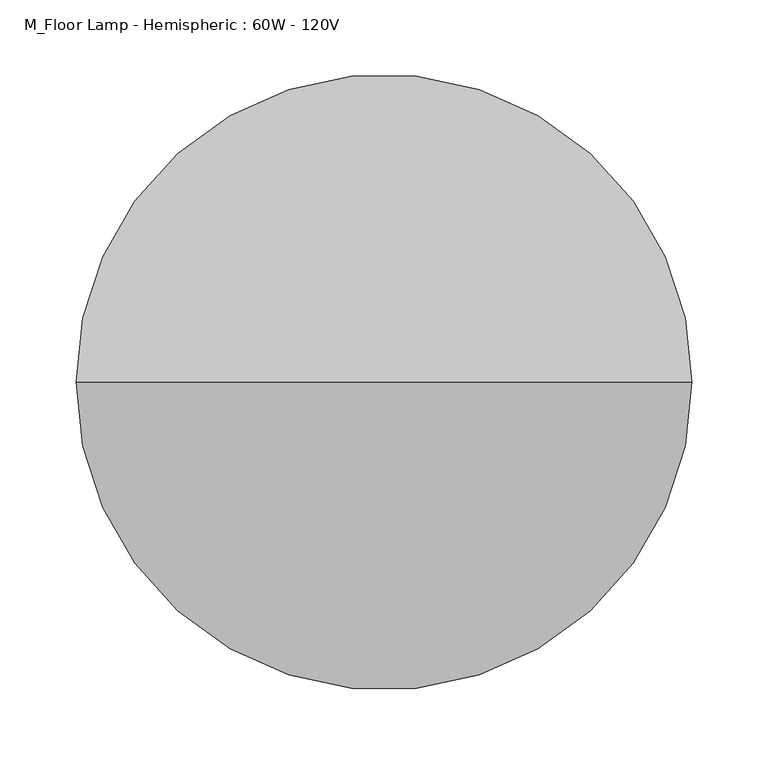
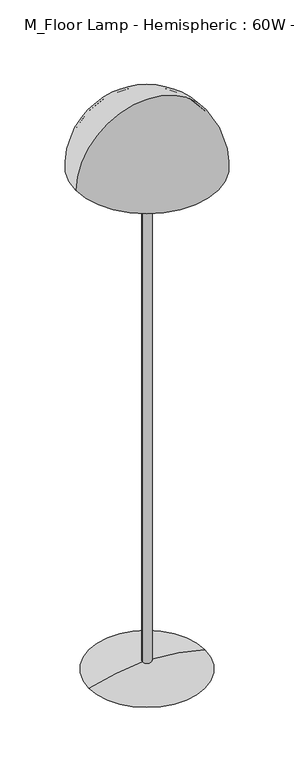
"""IFC4 building model written with IfcOpenShell, lengths in millimetres: light fixture geometry, M_Floor Lamp - Hemispheric : 60W - 120V."""

from ifc_helpers import new_model, si_unit, point, frame, origin, origin_with_axes, origin_2d, place, context, project, spatial, polyline, circle_curve, ellipse_curve, trimmed, segment, composite_curve, outline, extrude, source, transform, mapped, element, save
from ifc_brep_helpers import plane_surface, revolved_surface, advanced_brep


def m_floor_lamp_hemispheric_60w_120v_4a08ccbb(model_context):
    return source(origin(), model_context, "Body", "SolidModel", [
        extrude(outline(composite_curve([segment(trimmed(circle_curve(origin_2d(), 12.7), [point((-12.7, 0.0))], [point((12.7, 0.0))], False, "CARTESIAN"), True, "CONTINUOUS"), segment(trimmed(circle_curve(origin_2d(), 12.7), [point((12.7, 0.0))], [point((-12.7, 0.0))], False, "CARTESIAN"), True, "CONTINUOUS")], self_intersect=False)), frame((0.0, 0.0, 25.4), z_axis=(0.0, 0.0, 1.0), x_axis=(1.0, 0.0, 0.0)), (0.0, 0.0, 1.0), 1524.0),
        advanced_brep(
        [(-165.1, 0.0, 0.0), (165.1, 0.0, 0.0), (12.7, 0.0, 0.0), (-12.7, 0.0, 0.0), (-12.7, 0.0, 25.4), (12.7, 0.0, 25.4)],
        [
            (0, 1, circle_curve(frame((0.0, 0.0, 0.0), z_axis=(0.0, 0.0, -1.0), x_axis=(1.0, 0.0, 0.0)), 165.1)),
            (1, 2),
            (2, 3, circle_curve(origin_with_axes(), 12.7)),
            (3, 0),
            (1, 0, circle_curve(frame((0.0, 0.0, 0.0), z_axis=(0.0, 0.0, -1.0), x_axis=(1.0, 0.0, 0.0)), 165.1)),
            (3, 2, circle_curve(origin_with_axes(), 12.7)),
            (4, 5, circle_curve(frame((0.0, 0.0, 25.4), z_axis=(0.0, 0.0, -1.0), x_axis=(1.0, 0.0, 0.0)), 12.7)),
            (5, 1, circle_curve(frame((-10.5405788, 0.0, -583.9434729), z_axis=(0.0, 1.0, 0.0), x_axis=(1.0, 0.0, 0.0)), 609.7865138)),
            (0, 4, circle_curve(frame((10.5405788, 0.0, -583.9434729), z_axis=(0.0, 1.0, 0.0), x_axis=(-1.0, 0.0, 0.0)), 609.7865138)),
            (5, 4, circle_curve(frame((0.0, 0.0, 25.4), z_axis=(0.0, 0.0, -1.0), x_axis=(1.0, 0.0, 0.0)), 12.7)),
            (2, 5),
            (4, 3),
        ],
        [
            plane_surface(frame((0.0, 0.0, 0.0), z_axis=(0.0, 0.0, -1.0), x_axis=(1.0, 0.0, 0.0))),
            revolved_surface(trimmed(ellipse_curve(frame((-10.5405788, 0.0, -583.9434729), z_axis=(0.0, -1.0, 0.0), x_axis=(1.0, 0.0, 0.0)), 609.7865138, 609.7865138), [point((165.1, 0.0, 0.0))], [point((12.7, 0.0, 25.4))], True, "CARTESIAN"), (0.0, 0.0, 127.0), (0.0, 0.0, 1.0)),
            revolved_surface(polyline([(12.7, 0.0, 25.400000000000006), (12.7, 0.0, 0.0)]), (0.0, 0.0, 127.0), (0.0, 0.0, 1.0)),
        ],
        [
            (0, [[1, 2, 3, 4]]),
            (0, [[5, -4, 6, -2]]),
            (1, [[7, 8, -1, 9]]),
            (1, [[10, -9, -5, -8]]),
            (2, [[-3, 11, -7, 12]]),
            (2, [[-6, -12, -10, -11]]),
        ],
    ),
        advanced_brep(
        [(-197.591573, 0.0, 1510.4133868), (197.591573, 0.0, 1510.4133868), (0.0, 0.0, 1707.4075084), (-202.3305676, 0.0, 1510.4133868), (202.3305676, 0.0, 1510.4133868), (0.0, 0.0, 1713.4837615)],
        [
            (0, 1, circle_curve(frame((0.0, 0.0, 1510.4133868), z_axis=(0.0, 0.0, -1.0), x_axis=(1.0, 0.0, 0.0)), 197.591573)),
            (1, 2, circle_curve(frame((0.7416268, 0.0, 1510.5589055), z_axis=(0.0, -1.0, 0.0), x_axis=(1.0, 0.0, 0.0)), 196.85)),
            (2, 0, circle_curve(frame((-0.7416268, 0.0, 1510.5589055), z_axis=(0.0, -1.0, 0.0), x_axis=(-1.0, 0.0, 0.0)), 196.85)),
            (1, 0, circle_curve(frame((0.0, 0.0, 1510.4133868), z_axis=(0.0, 0.0, -1.0), x_axis=(1.0, 0.0, 0.0)), 197.591573)),
            (3, 4, circle_curve(frame((0.0, 0.0, 1510.4133868), z_axis=(0.0, 0.0, -1.0), x_axis=(1.0, 0.0, 0.0)), 202.3305676)),
            (4, 1),
            (0, 3),
            (4, 3, circle_curve(frame((0.0, 0.0, 1510.4133868), z_axis=(0.0, 0.0, -1.0), x_axis=(1.0, 0.0, 0.0)), 202.3305676)),
            (5, 4, circle_curve(frame((-0.8693923, 0.0, 1510.2856214), z_axis=(0.0, 1.0, 0.0), x_axis=(1.0, 0.0, 0.0)), 203.2)),
            (3, 5, circle_curve(frame((0.8693923, 0.0, 1510.2856214), z_axis=(0.0, 1.0, 0.0), x_axis=(-1.0, 0.0, 0.0)), 203.2)),
        ],
        [
            revolved_surface(trimmed(ellipse_curve(frame((0.7416268, 0.0, 1510.5589055), z_axis=(0.0, 1.0, 0.0), x_axis=(1.0, 0.0, 0.0)), 196.85, 196.85), [point((0.0, 0.0, 1707.4075084))], [point((197.591573, 0.0, 1510.4133868))], True, "CARTESIAN"), (0.0, 0.0, 1815.2133868), (0.0, 0.0, 1.0)),
            plane_surface(frame((0.0, 0.0, 1510.4133868), z_axis=(0.0, 0.0, -1.0), x_axis=(1.0, 0.0, 0.0))),
            revolved_surface(trimmed(ellipse_curve(frame((-0.8693923, 0.0, 1510.2856214), z_axis=(0.0, -1.0, 0.0), x_axis=(1.0, 0.0, 0.0)), 203.2, 203.2), [point((202.3305676, 0.0, 1510.4133868))], [point((0.0, 0.0, 1713.4837615))], True, "CARTESIAN"), (0.0, 0.0, 1815.2133868), (0.0, 0.0, 1.0)),
        ],
        [
            (0, [[1, 2, 3]]),
            (0, [[4, -3, -2]]),
            (1, [[5, 6, -1, 7]]),
            (1, [[8, -7, -4, -6]]),
            (2, [[9, -5, 10]]),
            (2, [[-10, -8, -9]]),
        ],
    ),
    ])


if __name__ == "__main__":
    model = new_model("IFC4")
    model_context = context("Model", 3, world=origin())
    ifc_project = project(units=[si_unit("LENGTHUNIT", "METRE", prefix="MILLI")], contexts=[model_context])
    site = spatial("IfcSite", under=ifc_project)
    building = spatial("IfcBuilding", under=site)
    placement = place(None, origin())
    m_floor_lamp_hemispheric_60w_120v_shape = m_floor_lamp_hemispheric_60w_120v_4a08ccbb(model_context)
    element("IfcLightFixture", 1, ObjectType="M_Floor Lamp - Hemispheric : 60W - 120V", at=placement, inside=building, context=model_context, shape_type="MappedRepresentation", body=[
        mapped(m_floor_lamp_hemispheric_60w_120v_shape, transform((0.0, 0.0, 0.0), x_axis=(1.0, 0.0, 0.0), y_axis=(0.0, 1.0, 0.0), z_axis=(0.0, 0.0, 1.0))),
    ])
    save(model, "model.ifc")

# Revit data of these elements
# Type "M_Floor Lamp - Hemispheric : 60W - 120V"
#   Photometric Web File = "CLFR1A19.ies"
#   Assembly Code = "D5020220"
#   Lamp = "A-19"
#   Wattage Comments = "60"
#   Wattage = 500 W
#   built-in parameter 1150110 = 2 (stored number, unit not read)
#   built-in parameter 1114217 = 4 (stored number, unit not read)
#   built-in parameter 1150109 = 2 (stored number, unit not read)
#   built-in parameter 1150113 = 1 (stored number, unit not read)
#   Tilt Angle = 90.00°
#   built-in parameter 1150115 = 1 (stored number, unit not read)
#   built-in parameter 1150105 = 3988.82 (stored number, unit not read)
#   built-in parameter 1150112 = 1 (stored number, unit not read)
#   built-in parameter 1150114 = 1 (stored number, unit not read)
#   built-in parameter 1150107 = 6500 (stored number, unit not read)
#   built-in parameter 1150106 = 39.8882 (stored number, unit not read)
#   built-in parameter 1150104 = 9.31353 (stored number, unit not read)
#   Ballast Voltage = 120 V
#   built-in parameter 1114218 = 1 (stored number, unit not read)
#   built-in parameter 1150133 = 10 (stored number, unit not read)
#   Lumens = 50125 lm
#   Apparent Load = 60 VA
#   built-in parameter 1150134 = 1
#   built-in parameter 1150137 = 1
#   Color Filter = 16777215
#   Ballast Number of Poles = 1
#   Stand = Steel, Chrome Plated
#   Shade = Glass, Frosted
#   Dimming Lamp Color Temperature Shift = (empty or 0)
#   Default Elevation = 0
# Element 1 (IfcLightFixture, "M_Floor Lamp - Hemispheric : 60W - 120V")
#   Materials on its faces: "Steel, Chrome Plated", "Glass, Frosted"
# Materials
#   "Steel, Chrome Plated": class "Metal", colour RGB 17 17 17, transparency 0, Description = "Chromiuim plated steel", Cost = 0
#   "Glass, Frosted": class "Glass", colour RGB 249 250 249, transparency 0.8, Description = "physical material", Cost = 0
